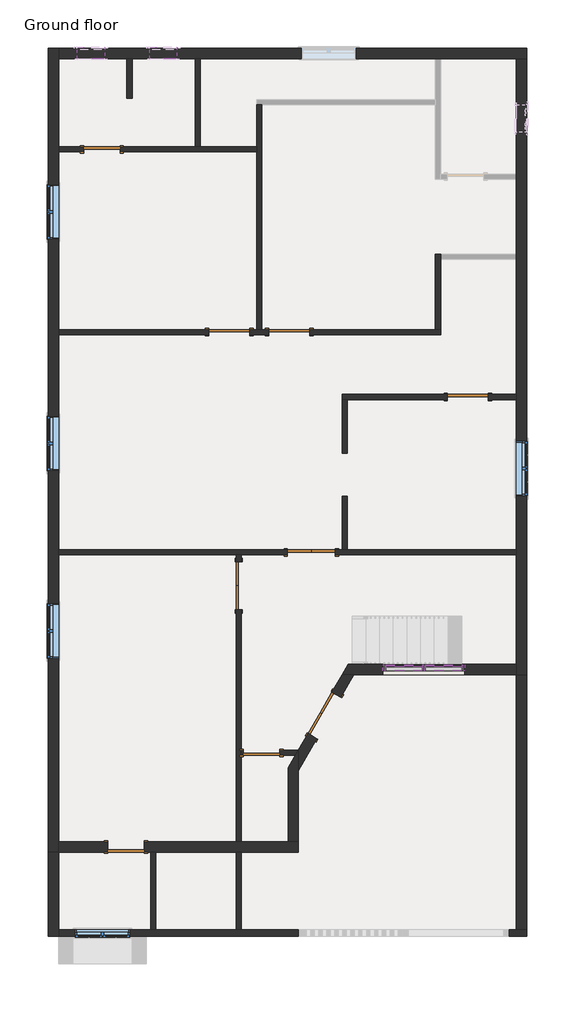
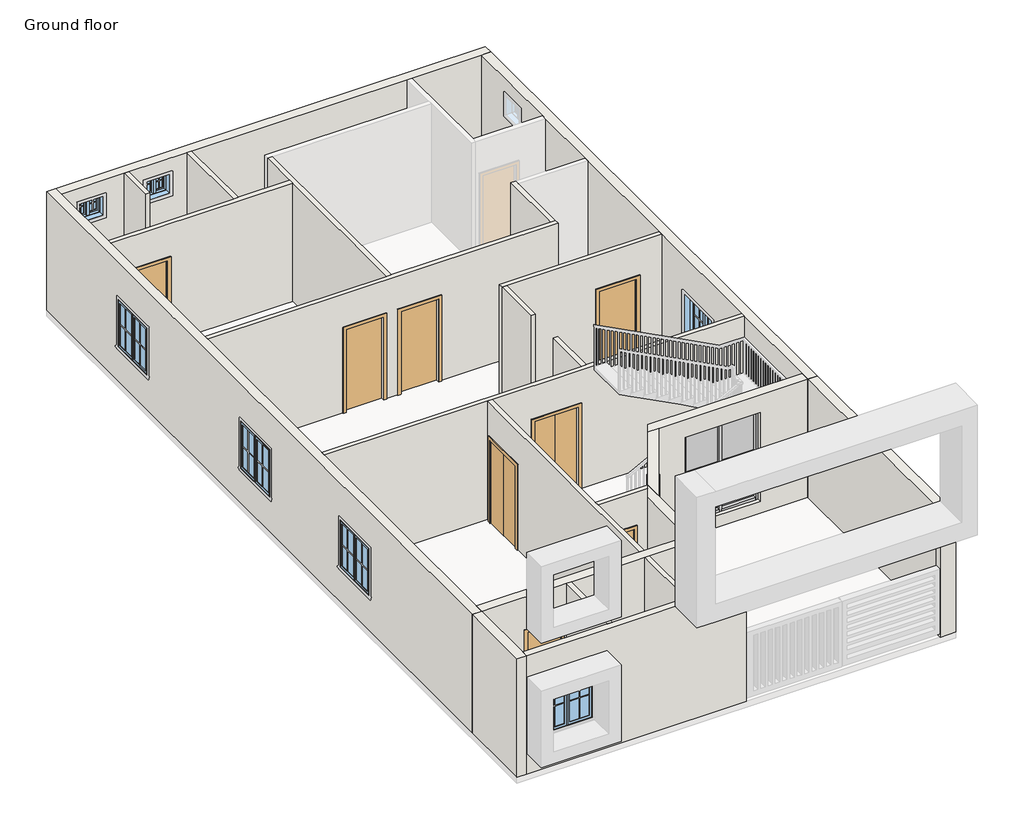
# One storey, part 1 of 3: 25 walls, 12 members, 9 doors, 7 windows, 4 plates.
"""IFC4 building model written with IfcOpenShell, lengths in millimetres."""

from ifc_helpers import new_model, si_unit, origin, origin_with_axes, place, context, project, spatial, polyline, outline, extrude, faceted_brep, transform, mapped, element, save
from components import door_d52489d9, door_d57fbbae, door_38851409, door_7b345704, single_flush_3_x7_e5f9f3c4, single_flush_3_x7_305aa2a5, member_c17f1be2, member_ad567e07, member_2b49869a, member_a715cb85, member_75074519, member_c4de40ee, system_panel_glazed_f4fd55f0, system_panel_glazed_231200ce, window_79894727, window_casement_double_4_x4_af3140d2, window_casement_double_4_x4_191d0cfb

model = new_model("IFC4")

# Units and contexts
model_context = context("Model", 3, world=origin())
ifc_project = project(units=[si_unit("LENGTHUNIT", "METRE", prefix="MILLI")], contexts=[model_context])

# Site, building, storey
site = spatial("IfcSite", under=ifc_project)
building = spatial("IfcBuilding", under=site)
storey = spatial("IfcBuildingStorey", under=building, Name="Ground floor", Elevation=0.0)

# Doors
placement = place(None, origin())
door_shape = door_d52489d9(model_context)
element("IfcDoor", 1, ObjectType="Door-Double-Flush_Panel : 3'6\"X7'", at=placement, inside=storey, context=model_context, shape_type="MappedRepresentation", body=[
    mapped(door_shape, transform((388.5194418, -4721.06525, 0.0), x_axis=(0.5010362705417002, 0.8654262854811288, 0.0), y_axis=(-0.8654262854811288, 0.5010362705417002, 0.0), z_axis=(0.0, 0.0, 1.0))),
])
door_2_shape = door_d57fbbae(model_context)
element("IfcDoor", 2, ObjectType="Door-Double-Flush_Panel : 3'6\"X7'", at=placement, inside=storey, context=model_context, shape_type="MappedRepresentation", body=[
    mapped(door_2_shape, transform((96.8585096, -1088.0023906, 0.0), x_axis=(1.0, 0.0, 0.0), y_axis=(0.0, 1.0, 0.0), z_axis=(0.0, 0.0, 1.0))),
])
element("IfcDoor", 3, ObjectType="Door-Double-Flush_Panel : 3'6\"X7'", at=placement, inside=storey, context=model_context, shape_type="MappedRepresentation", body=[
    mapped(door_2_shape, transform((-1522.3914904, -1830.9523906, 0.0), x_axis=(0.0, 1.0, 0.0), y_axis=(-1.0, 0.0, 0.0), z_axis=(0.0, 0.0, 1.0))),
])
door_3_shape = door_38851409(model_context)
element("IfcDoor", 4, ObjectType="Single-Flush : 2'8\"X7'", at=placement, inside=storey, context=model_context, shape_type="MappedRepresentation", body=[
    mapped(door_3_shape, transform((-1014.3914904, -5558.4023906, 0.0), x_axis=(1.0, 0.0, 0.0), y_axis=(0.0, 1.0, 0.0), z_axis=(0.0, 0.0, 1.0))),
])
element("IfcDoor", 5, ObjectType="Single-Flush : 2'8\"X7'", at=placement, inside=storey, context=model_context, shape_type="MappedRepresentation", body=[
    mapped(door_3_shape, transform((-4576.7414904, 7903.5976094, 0.0), x_axis=(-1.0, 0.0, 0.0), y_axis=(0.0, -1.0, 0.0), z_axis=(0.0, 0.0, 1.0))),
])
door_4_shape = door_7b345704(model_context)
element("IfcDoor", 6, ObjectType="Single-Flush : 2'8\"X7'", at=placement, inside=storey, context=model_context, shape_type="MappedRepresentation", body=[
    mapped(door_4_shape, transform((-4036.9914904, -7660.2523906, 0.0), x_axis=(1.0, 0.0, 0.0), y_axis=(0.0, 1.0, 0.0), z_axis=(0.0, 0.0, 1.0))),
])
single_flush_3_x7_shape = single_flush_3_x7_e5f9f3c4(model_context)
element("IfcDoor", 7, ObjectType="Single-Flush : 3'X7'", at=placement, inside=storey, context=model_context, shape_type="MappedRepresentation", body=[
    mapped(single_flush_3_x7_shape, transform((-1731.9414904, 3826.8976094, 0.0), x_axis=(1.0, 0.0, 0.0), y_axis=(0.0, 1.0, 0.0), z_axis=(0.0, 0.0, 1.0))),
])
single_flush_3_x7_2_shape = single_flush_3_x7_305aa2a5(model_context)
element("IfcDoor", 8, ObjectType="Single-Flush : 3'X7'", at=placement, inside=storey, context=model_context, shape_type="MappedRepresentation", body=[
    mapped(single_flush_3_x7_2_shape, transform((-398.4414904, 3826.8976094, 0.0), x_axis=(-1.0, 0.0, 0.0), y_axis=(0.0, -1.0, 0.0), z_axis=(0.0, 0.0, 1.0))),
])
element("IfcDoor", 9, ObjectType="Single-Flush : 3'X7'", at=placement, inside=storey, context=model_context, shape_type="MappedRepresentation", body=[
    mapped(single_flush_3_x7_2_shape, transform((3589.3585096, 2379.0976094, 0.0), x_axis=(-1.0, 0.0, 0.0), y_axis=(0.0, -1.0, 0.0), z_axis=(0.0, 0.0, 1.0))),
])

# Members
member_shape = member_c17f1be2(model_context)
element("IfcMember", 10, ObjectType="Rectangular Mullion : 2.5\" x 5\" rectangular", at=placement, inside=storey, context=model_context, shape_type="MappedRepresentation", body=[
    mapped(member_shape, transform((3456.0085096, -3659.7523906, 2590.8), x_axis=(0.0, 0.0, 1.0), y_axis=(0.0, -1.0, 0.0), z_axis=(1.0, 0.0, 0.0))),
])
element("IfcMember", 11, ObjectType="Rectangular Mullion : 2.5\" x 5\" rectangular", at=placement, inside=storey, context=model_context, shape_type="MappedRepresentation", body=[
    mapped(member_shape, transform((2573.3585096, -3659.7523906, 2590.8), x_axis=(0.0, 0.0, 1.0), y_axis=(0.0, -1.0, 0.0), z_axis=(1.0, 0.0, 0.0))),
])
element("IfcMember", 12, ObjectType="Rectangular Mullion : 2.5\" x 5\" rectangular", at=placement, inside=storey, context=model_context, shape_type="MappedRepresentation", body=[
    mapped(member_shape, transform((1754.2085096, -3659.7523906, 304.8), x_axis=(0.0, 0.0, -1.0), y_axis=(0.0, -1.0, 0.0), z_axis=(-1.0, 0.0, 0.0))),
])
element("IfcMember", 13, ObjectType="Rectangular Mullion : 2.5\" x 5\" rectangular", at=placement, inside=storey, context=model_context, shape_type="MappedRepresentation", body=[
    mapped(member_shape, transform((2636.8585096, -3659.7523906, 304.8), x_axis=(0.0, 0.0, -1.0), y_axis=(0.0, -1.0, 0.0), z_axis=(-1.0, 0.0, 0.0))),
])
member_2_shape = member_ad567e07(model_context)
element("IfcMember", 14, ObjectType="Rectangular Mullion : 2.5\" x 5\" rectangular", at=placement, inside=storey, context=model_context, shape_type="MappedRepresentation", body=[
    mapped(member_2_shape, transform((2573.3585096, -3659.7523906, 1524.0), x_axis=(0.0, 0.0, 1.0), y_axis=(0.0, -1.0, 0.0), z_axis=(1.0, 0.0, 0.0))),
])
element("IfcMember", 15, ObjectType="Rectangular Mullion : 2.5\" x 5\" rectangular", at=placement, inside=storey, context=model_context, shape_type="MappedRepresentation", body=[
    mapped(member_2_shape, transform((3456.0085096, -3659.7523906, 1524.0), x_axis=(0.0, 0.0, 1.0), y_axis=(0.0, -1.0, 0.0), z_axis=(1.0, 0.0, 0.0))),
])
member_3_shape = member_2b49869a(model_context)
element("IfcMember", 16, ObjectType="Rectangular Mullion : 2.5\" x 5\" rectangular", at=placement, inside=storey, context=model_context, shape_type="MappedRepresentation", body=[
    mapped(member_3_shape, transform((2605.1085096, -3659.7523906, 304.8), x_axis=(1.0, 0.0, 0.0), y_axis=(0.0, -1.0, 0.0), z_axis=(0.0, 0.0, -1.0))),
])
member_4_shape = member_a715cb85(model_context)
element("IfcMember", 17, ObjectType="Rectangular Mullion : 2.5\" x 5\" rectangular", at=placement, inside=storey, context=model_context, shape_type="MappedRepresentation", body=[
    mapped(member_4_shape, transform((2605.1085096, -3659.7523906, 1524.0), x_axis=(1.0, 0.0, 0.0), y_axis=(0.0, -1.0, 0.0), z_axis=(0.0, 0.0, -1.0))),
])
member_5_shape = member_75074519(model_context)
element("IfcMember", 18, ObjectType="Rectangular Mullion : 2.5\" x 5\" rectangular", at=placement, inside=storey, context=model_context, shape_type="MappedRepresentation", body=[
    mapped(member_5_shape, transform((3519.5085096, -3659.7523906, 304.8), x_axis=(1.0, 0.0, 0.0), y_axis=(0.0, -1.0, 0.0), z_axis=(0.0, 0.0, -1.0))),
])
member_6_shape = member_c4de40ee(model_context)
element("IfcMember", 19, ObjectType="Rectangular Mullion : 2.5\" x 5\" rectangular", at=placement, inside=storey, context=model_context, shape_type="MappedRepresentation", body=[
    mapped(member_6_shape, transform((1690.7085096, -3659.7523906, 2590.8), x_axis=(-1.0, 0.0, 0.0), y_axis=(0.0, -1.0, 0.0), z_axis=(0.0, 0.0, 1.0))),
])
element("IfcMember", 20, ObjectType="Rectangular Mullion : 2.5\" x 5\" rectangular", at=placement, inside=storey, context=model_context, shape_type="MappedRepresentation", body=[
    mapped(member_6_shape, transform((3519.5085096, -3659.7523906, 1524.0), x_axis=(1.0, 0.0, 0.0), y_axis=(0.0, -1.0, 0.0), z_axis=(0.0, 0.0, -1.0))),
])
element("IfcMember", 21, ObjectType="Rectangular Mullion : 2.5\" x 5\" rectangular", at=placement, inside=storey, context=model_context, shape_type="MappedRepresentation", body=[
    mapped(member_5_shape, transform((1690.7085096, -3659.7523906, 1524.0), x_axis=(-1.0, 0.0, 0.0), y_axis=(0.0, -1.0, 0.0), z_axis=(0.0, 0.0, 1.0))),
])

# Plates
system_panel_glazed_shape = system_panel_glazed_f4fd55f0(model_context)
element("IfcPlate", 22, ObjectType="System Panel : Glazed", at=placement, inside=storey, context=model_context, shape_type="MappedRepresentation", body=[
    mapped(system_panel_glazed_shape, transform((2163.7835096, -3659.7523906, 1555.75), x_axis=(1.0, 0.0, 0.0), y_axis=(0.0, 1.0, 0.0), z_axis=(0.0, 0.0, 1.0))),
])
element("IfcPlate", 23, ObjectType="System Panel : Glazed", at=placement, inside=storey, context=model_context, shape_type="MappedRepresentation", body=[
    mapped(system_panel_glazed_shape, transform((3046.4335096, -3659.7523906, 1555.75), x_axis=(1.0, 0.0, 0.0), y_axis=(0.0, 1.0, 0.0), z_axis=(0.0, 0.0, 1.0))),
])
system_panel_glazed_2_shape = system_panel_glazed_231200ce(model_context)
element("IfcPlate", 24, ObjectType="System Panel : Glazed", at=placement, inside=storey, context=model_context, shape_type="MappedRepresentation", body=[
    mapped(system_panel_glazed_2_shape, transform((2163.7835096, -3659.7523906, 368.3), x_axis=(1.0, 0.0, 0.0), y_axis=(0.0, 1.0, 0.0), z_axis=(0.0, 0.0, 1.0))),
])
element("IfcPlate", 25, ObjectType="System Panel : Glazed", at=placement, inside=storey, context=model_context, shape_type="MappedRepresentation", body=[
    mapped(system_panel_glazed_2_shape, transform((3046.4335096, -3659.7523906, 368.3), x_axis=(1.0, 0.0, 0.0), y_axis=(0.0, 1.0, 0.0), z_axis=(0.0, 0.0, 1.0))),
])

# Walls
element("IfcWall", 26, ObjectType="4.5\"", at=placement, inside=storey, context=model_context, shape_type="Brep", body=[
    faceted_brep([(-5543.5289904, 7846.4476094, 0.0), (-4983.1414904, 7846.4476094, 0.0), (-4983.1414904, 7846.4476094, 2133.6), (-4170.3414904, 7846.4476094, 2133.6), (-4170.3414904, 7846.4476094, 0.0), (-1122.3414904, 7846.4476094, 0.0), (-1122.3414904, 7846.4476094, 3048.0), (-5543.5289904, 7846.4476094, 3048.0), (-4983.1414904, 7960.7476094, 2133.6), (-4983.1414904, 7960.7476094, 0.0), (-5543.5289904, 7960.7476094, 0.0), (-5543.5289904, 7960.7476094, 3048.0), (-2493.9414904, 7960.7476094, 3048.0), (-2379.6414904, 7960.7476094, 3048.0), (-1122.3414904, 7960.7476094, 3048.0), (-1122.3414904, 7960.7476094, 0.0), (-2379.6414904, 7960.7476094, 0.0), (-2493.9414904, 7960.7476094, 0.0), (-4170.3414904, 7960.7476094, 0.0), (-4170.3414904, 7960.7476094, 2133.6)], [[[0, 1, 2, 3, 4, 5, 6, 7]], [[8, 9, 10, 11, 12, 13, 14, 15, 16, 17, 18, 19]], [[10, 9, 1, 0]], [[18, 17, 16, 15, 5, 4]], [[7, 6, 14, 13, 12, 11]], [[0, 7, 11, 10]], [[6, 5, 15, 14]], [[2, 1, 9, 8]], [[3, 2, 8, 19]], [[4, 3, 19, 18]]]),
])
element("IfcWall", 27, ObjectType="4.5\"", at=placement, inside=storey, context=model_context, shape_type="SweptSolid", body=[
    extrude(outline(polyline([(-2493.9414904, 7960.7476094), (-2493.9414904, 9929.2476094), (-2379.6414904, 9929.2476094), (-2379.6414904, 7960.7476094), (-2493.9414904, 7960.7476094)])), origin_with_axes(), (0.0, 0.0, 1.0), 3048.0),
])
element("IfcWall", 28, ObjectType="4.5\"", at=placement, inside=storey, context=model_context, shape_type="SweptSolid", body=[
    extrude(outline(polyline([(-4017.9414904, 9045.2567445), (-4017.9414904, 9929.2476094), (-3903.6414904, 9929.2476094), (-3903.6414904, 9045.2567445), (-4017.9414904, 9045.2567445)])), origin_with_axes(), (0.0, 0.0, 1.0), 3048.0),
])
element("IfcWall", 29, ObjectType="4.5\"", at=placement, inside=storey, context=model_context, shape_type="Brep", body=[
    faceted_brep([(-1274.7414904, 3769.7476094, 0.0), (-855.6414904, 3769.7476094, 0.0), (-855.6414904, 3769.7476094, 2133.6), (58.7585096, 3769.7476094, 2133.6), (58.7585096, 3769.7476094, 0.0), (2979.7585096, 3769.7476094, 0.0), (2979.7585096, 3769.7476094, 3048.0), (-5543.5289904, 3769.7476094, 3048.0), (-5543.5289904, 3769.7476094, 0.0), (-2189.1414904, 3769.7476094, 0.0), (-2189.1414904, 3769.7476094, 2133.6), (-1274.7414904, 3769.7476094, 2133.6), (-855.6414904, 3884.0476094, 2133.6), (-855.6414904, 3884.0476094, 0.0), (-1008.0414904, 3884.0476094, 0.0), (-1122.3414904, 3884.0476094, 0.0), (-1274.7414904, 3884.0476094, 0.0), (-1274.7414904, 3884.0476094, 2133.6), (-2189.1414904, 3884.0476094, 2133.6), (-2189.1414904, 3884.0476094, 0.0), (-5543.5289904, 3884.0476094, 0.0), (-5543.5289904, 3884.0476094, 3048.0), (-1122.3414904, 3884.0476094, 3048.0), (-1008.0414904, 3884.0476094, 3048.0), (2865.4585096, 3884.0476094, 3048.0), (2979.7585096, 3884.0476094, 3048.0), (2979.7585096, 3884.0476094, 0.0), (2865.4585096, 3884.0476094, 0.0), (58.7585096, 3884.0476094, 0.0), (58.7585096, 3884.0476094, 2133.6)], [[[0, 1, 2, 3, 4, 5, 6, 7, 8, 9, 10, 11]], [[12, 13, 14, 15, 16, 17, 18, 19, 20, 21, 22, 23, 24, 25, 26, 27, 28, 29]], [[9, 8, 20, 19]], [[28, 27, 26, 5, 4]], [[16, 15, 14, 13, 1, 0]], [[7, 6, 25, 24, 23, 22, 21]], [[8, 7, 21, 20]], [[6, 5, 26, 25]], [[17, 16, 0, 11]], [[18, 17, 11, 10]], [[19, 18, 10, 9]], [[2, 1, 13, 12]], [[3, 2, 12, 29]], [[4, 3, 29, 28]]]),
])
element("IfcWall", 30, ObjectType="4.5\"", at=placement, inside=storey, context=model_context, shape_type="Brep", body=[
    faceted_brep([(2979.7585096, 3884.0476094, 0.0), (2979.7585096, 5446.1476094, 0.0), (2979.7585096, 5560.4476094, 0.0), (2979.7585096, 5560.4476094, 3048.0), (2979.7585096, 5446.1476094, 3048.0), (2979.7585096, 3884.0476094, 3048.0), (2865.4585096, 3884.0476094, 0.0), (2865.4585096, 3884.0476094, 3048.0), (2865.4585096, 5560.4476094, 3048.0), (2865.4585096, 5560.4476094, 0.0)], [[[0, 1, 2, 3, 4, 5]], [[6, 7, 8, 9]], [[2, 1, 0, 6, 9]], [[5, 4, 3, 8, 7]], [[0, 5, 7, 6]], [[3, 2, 9, 8]]]),
])
element("IfcWall", 31, ObjectType="4.5\"", at=placement, inside=storey, context=model_context, shape_type="Brep", body=[
    faceted_brep([(3132.1585096, 2436.2476094, 2133.6), (3132.1585096, 2436.2476094, 0.0), (782.6585096, 2436.2476094, 0.0), (782.6585096, 2436.2476094, 3048.0), (4668.8585096, 2436.2476094, 3048.0), (4668.8585096, 2436.2476094, 0.0), (4046.5585096, 2436.2476094, 0.0), (4046.5585096, 2436.2476094, 2133.6), (782.6585096, 2321.9476094, 0.0), (896.9585096, 2321.9476094, 0.0), (3132.1585096, 2321.9476094, 0.0), (3132.1585096, 2321.9476094, 2133.6), (4046.5585096, 2321.9476094, 2133.6), (4046.5585096, 2321.9476094, 0.0), (4668.8585096, 2321.9476094, 0.0), (4668.8585096, 2321.9476094, 3048.0), (896.9585096, 2321.9476094, 3048.0), (782.6585096, 2321.9476094, 3048.0)], [[[0, 1, 2, 3, 4, 5, 6, 7]], [[8, 9, 10, 11, 12, 13, 14, 15, 16, 17]], [[6, 5, 14, 13]], [[2, 1, 10, 9, 8]], [[4, 3, 17, 16, 15]], [[5, 4, 15, 14]], [[3, 2, 8, 17]], [[11, 10, 1, 0]], [[12, 11, 0, 7]], [[13, 12, 7, 6]]]),
])
element("IfcWall", 32, ObjectType="4.5\"", at=placement, inside=storey, context=model_context, shape_type="SweptSolid", body=[
    extrude(outline(polyline([(782.6585096, 1121.7976094), (782.6585096, 2321.9476094), (896.9585096, 2321.9476094), (896.9585096, 1121.7976094), (782.6585096, 1121.7976094)])), origin_with_axes(), (0.0, 0.0, 1.0), 3048.0),
])
element("IfcWall", 33, ObjectType="4.5\"", at=placement, inside=storey, context=model_context, shape_type="Brep", body=[
    faceted_brep([(4668.8585096, -1145.1523906, 3048.0), (-1465.2414904, -1145.1523906, 3048.0), (-1579.5414904, -1145.1523906, 3048.0), (-5543.5289904, -1145.1523906, 3048.0), (-5543.5289904, -1145.1523906, 0.0), (-1579.5414904, -1145.1523906, 0.0), (-1465.2414904, -1145.1523906, 0.0), (-436.5414904, -1145.1523906, 0.0), (-436.5414904, -1145.1523906, 2133.6), (630.2585096, -1145.1523906, 2133.6), (630.2585096, -1145.1523906, 0.0), (4668.8585096, -1145.1523906, 0.0), (-5543.5289904, -1030.8523906, 3048.0), (782.6585096, -1030.8523906, 3048.0), (896.9585096, -1030.8523906, 3048.0), (4668.8585096, -1030.8523906, 3048.0), (4668.8585096, -1030.8523906, 0.0), (896.9585096, -1030.8523906, 0.0), (782.6585096, -1030.8523906, 0.0), (630.2585096, -1030.8523906, 0.0), (630.2585096, -1030.8523906, 2133.6), (-436.5414904, -1030.8523906, 2133.6), (-436.5414904, -1030.8523906, 0.0), (-5543.5289904, -1030.8523906, 0.0)], [[[0, 1, 2, 3, 4, 5, 6, 7, 8, 9, 10, 11]], [[12, 13, 14, 15, 16, 17, 18, 19, 20, 21, 22, 23]], [[4, 23, 22, 7, 6, 5]], [[16, 11, 10, 19, 18, 17]], [[3, 2, 1, 0, 15, 14, 13, 12]], [[4, 3, 12, 23]], [[0, 11, 16, 15]], [[9, 20, 19, 10]], [[20, 9, 8, 21]], [[21, 8, 7, 22]]]),
])
element("IfcWall", 34, ObjectType="4.5\"", at=placement, inside=storey, context=model_context, shape_type="Brep", body=[
    faceted_brep([(-1579.5414904, -7545.9523906, 3048.0), (-1579.5414904, -1145.1523906, 3048.0), (-1579.5414904, -1145.1523906, 0.0), (-1579.5414904, -1297.5523906, 0.0), (-1579.5414904, -1297.5523906, 2133.6), (-1579.5414904, -2364.3523906, 2133.6), (-1579.5414904, -2364.3523906, 0.0), (-1579.5414904, -7545.9523906, 0.0), (-1465.2414904, -1145.1523906, 3048.0), (-1465.2414904, -5501.2523906, 3048.0), (-1465.2414904, -5615.5523906, 3048.0), (-1465.2414904, -7545.9523906, 3048.0), (-1465.2414904, -7545.9523906, 0.0), (-1465.2414904, -5615.5523906, 0.0), (-1465.2414904, -5501.2523906, 0.0), (-1465.2414904, -2364.3523906, 0.0), (-1465.2414904, -2364.3523906, 2133.6), (-1465.2414904, -1297.5523906, 2133.6), (-1465.2414904, -1297.5523906, 0.0), (-1465.2414904, -1145.1523906, 0.0)], [[[0, 1, 2, 3, 4, 5, 6, 7]], [[8, 9, 10, 11, 12, 13, 14, 15, 16, 17, 18, 19]], [[2, 19, 18, 3]], [[12, 7, 6, 15, 14, 13]], [[1, 0, 11, 10, 9, 8]], [[0, 7, 12, 11]], [[2, 1, 8, 19]], [[17, 4, 3, 18]], [[4, 17, 16, 5]], [[5, 16, 15, 6]]]),
])
element("IfcWall", 35, ObjectType="4.5\"", at=placement, inside=storey, context=model_context, shape_type="Brep", body=[
    faceted_brep([(-607.9914904, -5615.5523906, 2133.6), (-607.9914904, -5615.5523906, 0.0), (-261.4151747, -5615.5523906, 0.0), (-261.4151747, -5615.5523906, 3048.0), (-1465.2414904, -5615.5523906, 3048.0), (-1465.2414904, -5615.5523906, 0.0), (-1420.7914904, -5615.5523906, 0.0), (-1420.7914904, -5615.5523906, 2133.6), (-195.2414904, -5501.2523906, 0.0), (-607.9914904, -5501.2523906, 0.0), (-607.9914904, -5501.2523906, 2133.6), (-1420.7914904, -5501.2523906, 2133.6), (-1420.7914904, -5501.2523906, 0.0), (-1465.2414904, -5501.2523906, 0.0), (-1465.2414904, -5501.2523906, 3048.0), (-195.2414904, -5501.2523906, 3048.0)], [[[0, 1, 2, 3, 4, 5, 6, 7]], [[8, 9, 10, 11, 12, 13, 14, 15]], [[6, 5, 13, 12]], [[2, 1, 9, 8]], [[4, 3, 15, 14]], [[3, 2, 8, 15]], [[5, 4, 14, 13]], [[10, 9, 1, 0]], [[11, 10, 0, 7]], [[12, 11, 7, 6]]]),
])
element("IfcWall", 36, ObjectType="4.5\"", at=placement, inside=storey, context=model_context, shape_type="Brep", body=[
    faceted_brep([(-1122.3414904, 8900.5476094, 0.0), (-1122.3414904, 7960.7476094, 0.0), (-1122.3414904, 7846.4476094, 0.0), (-1122.3414904, 3884.0476094, 0.0), (-1122.3414904, 3884.0476094, 3048.0), (-1122.3414904, 7846.4476094, 3048.0), (-1122.3414904, 7960.7476094, 3048.0), (-1122.3414904, 8900.5476094, 3048.0), (-1008.0414904, 8900.5476094, 0.0), (-1008.0414904, 8900.5476094, 3048.0), (-1008.0414904, 3884.0476094, 3048.0), (-1008.0414904, 3884.0476094, 0.0)], [[[0, 1, 2, 3, 4, 5, 6, 7]], [[8, 9, 10, 11]], [[3, 2, 1, 0, 8, 11]], [[7, 6, 5, 4, 10, 9]], [[0, 7, 9, 8]], [[4, 3, 11, 10]]]),
])
element("IfcWall", 37, ObjectType="4.5\"", at=placement, inside=storey, context=model_context, shape_type="SweptSolid", body=[
    extrude(outline(polyline([(-3484.5414904, -9501.7523906), (-3484.5414904, -7774.5523906), (-3370.2414904, -7774.5523906), (-3370.2414904, -9501.7523906), (-3484.5414904, -9501.7523906)])), origin_with_axes(), (0.0, 0.0, 1.0), 3048.0),
])
element("IfcWall", 38, ObjectType="4.5\"", at=placement, inside=storey, context=model_context, shape_type="SweptSolid", body=[
    extrude(outline(polyline([(-1579.5414904, -9501.7523906), (-1579.5414904, -7774.5523906), (-1465.2414904, -7774.5523906), (-1465.2414904, -9501.7523906), (-1579.5414904, -9501.7523906)])), origin_with_axes(), (0.0, 0.0, 1.0), 3048.0),
])
element("IfcWall", 39, ObjectType="4.5\"", at=placement, inside=storey, context=model_context, shape_type="SweptSolid", body=[
    extrude(outline(polyline([(782.6585096, -1030.8523906), (782.6585096, 169.2976094), (896.9585096, 169.2976094), (896.9585096, -1030.8523906), (782.6585096, -1030.8523906)])), origin_with_axes(), (0.0, 0.0, 1.0), 3048.0),
])
element("IfcWall", 40, ObjectType="6\"", at=placement, inside=storey, context=model_context, shape_type="Brep", body=[
    faceted_brep([(-5543.5289904, -9654.1523906, 0.0), (-195.2414904, -9654.1523906, 0.0), (-195.2414904, -9654.1523906, 3048.0), (-5543.5289904, -9654.1523906, 3048.0), (-5171.2602404, -9654.1523906, 2133.6), (-3952.0602404, -9654.1523906, 2133.6), (-3952.0602404, -9654.1523906, 914.4), (-5171.2602404, -9654.1523906, 914.4), (-5543.5289904, -9501.7523906, 0.0), (-5543.5289904, -9501.7523906, 3048.0), (-3484.5414904, -9501.7523906, 3048.0), (-3370.2414904, -9501.7523906, 3048.0), (-1579.5414904, -9501.7523906, 3048.0), (-1465.2414904, -9501.7523906, 3048.0), (-195.2414904, -9501.7523906, 3048.0), (-195.2414904, -9501.7523906, 0.0), (-1465.2414904, -9501.7523906, 0.0), (-1579.5414904, -9501.7523906, 0.0), (-3370.2414904, -9501.7523906, 0.0), (-3484.5414904, -9501.7523906, 0.0), (-5171.2602404, -9501.7523906, 2133.6), (-5171.2602404, -9501.7523906, 914.4), (-3952.0602404, -9501.7523906, 914.4), (-3952.0602404, -9501.7523906, 2133.6)], [[[0, 1, 2, 3], [4, 5, 6, 7]], [[8, 9, 10, 11, 12, 13, 14, 15, 16, 17, 18, 19], [20, 21, 22, 23]], [[1, 0, 8, 19, 18, 17, 16, 15]], [[2, 1, 15, 14]], [[3, 2, 14, 13, 12, 11, 10, 9]], [[0, 3, 9, 8]], [[21, 20, 4, 7]], [[22, 21, 7, 6]], [[23, 22, 6, 5]], [[20, 23, 5, 4]]]),
])
element("IfcWall", 41, ObjectType="6\"", at=placement, inside=storey, context=model_context, shape_type="Brep", body=[
    faceted_brep([(4897.4585096, -9501.7523906, 0.0), (4668.8585096, -9501.7523906, 0.0), (4516.4585096, -9501.7523906, 0.0), (4516.4585096, -9501.7523906, 3048.0), (4668.8585096, -9501.7523906, 3048.0), (4897.4585096, -9501.7523906, 3048.0), (4897.4585096, -9654.1523906, 0.0), (4897.4585096, -9654.1523906, 3048.0), (4516.4585096, -9654.1523906, 3048.0), (4516.4585096, -9654.1523906, 0.0)], [[[0, 1, 2, 3, 4, 5]], [[6, 7, 8, 9]], [[2, 1, 0, 6, 9]], [[3, 2, 9, 8]], [[5, 4, 3, 8, 7]], [[0, 5, 7, 6]]]),
])
element("IfcWall", 42, ObjectType="9\" 2", at=placement, inside=storey, context=model_context, shape_type="Brep", body=[
    faceted_brep([(-5772.1289904, 10157.8476094, 0.0), (-5772.1289904, -7774.5523906, 0.0), (-5772.1289904, -7774.5523906, 3048.0), (-5772.1289904, 10157.8476094, 3048.0), (-5772.1289904, 7117.9239079, 2133.6), (-5772.1289904, 5898.7239079, 2133.6), (-5772.1289904, 5898.7239079, 914.4), (-5772.1289904, 7117.9239079, 914.4), (-5772.1289904, 1953.7982391, 2133.6), (-5772.1289904, 734.5982391, 2133.6), (-5772.1289904, 734.5982391, 914.4), (-5772.1289904, 1953.7982391, 914.4), (-5772.1289904, -2229.9627914, 2133.6), (-5772.1289904, -3449.1627914, 2133.6), (-5772.1289904, -3449.1627914, 914.4), (-5772.1289904, -2229.9627914, 914.4), (-5543.5289904, 10157.8476094, 0.0), (-5543.5289904, 10157.8476094, 3048.0), (-5543.5289904, 9929.2476094, 3048.0), (-5543.5289904, 7960.7476094, 3048.0), (-5543.5289904, 7846.4476094, 3048.0), (-5543.5289904, 3884.0476094, 3048.0), (-5543.5289904, 3769.7476094, 3048.0), (-5543.5289904, -1030.8523906, 3048.0), (-5543.5289904, -1145.1523906, 3048.0), (-5543.5289904, -7545.9523906, 3048.0), (-5543.5289904, -7774.5523906, 3048.0), (-5543.5289904, -7774.5523906, 0.0), (-5543.5289904, -7545.9523906, 0.0), (-5543.5289904, -1145.1523906, 0.0), (-5543.5289904, -1030.8523906, 0.0), (-5543.5289904, 3769.7476094, 0.0), (-5543.5289904, 3884.0476094, 0.0), (-5543.5289904, 7846.4476094, 0.0), (-5543.5289904, 7960.7476094, 0.0), (-5543.5289904, 9929.2476094, 0.0), (-5543.5289904, 7117.9239079, 2133.6), (-5543.5289904, 7117.9239079, 914.4), (-5543.5289904, 5898.7239079, 914.4), (-5543.5289904, 5898.7239079, 2133.6), (-5543.5289904, 1953.7982391, 2133.6), (-5543.5289904, 1953.7982391, 914.4), (-5543.5289904, 734.5982391, 914.4), (-5543.5289904, 734.5982391, 2133.6), (-5543.5289904, -2229.9627914, 2133.6), (-5543.5289904, -2229.9627914, 914.4), (-5543.5289904, -3449.1627914, 914.4), (-5543.5289904, -3449.1627914, 2133.6)], [[[0, 1, 2, 3], [4, 5, 6, 7], [8, 9, 10, 11], [12, 13, 14, 15]], [[16, 17, 18, 19, 20, 21, 22, 23, 24, 25, 26, 27, 28, 29, 30, 31, 32, 33, 34, 35], [36, 37, 38, 39], [40, 41, 42, 43], [44, 45, 46, 47]], [[1, 0, 16, 35, 34, 33, 32, 31, 30, 29, 28, 27]], [[3, 2, 26, 25, 24, 23, 22, 21, 20, 19, 18, 17]], [[2, 1, 27, 26]], [[0, 3, 17, 16]], [[37, 36, 4, 7]], [[38, 37, 7, 6]], [[39, 38, 6, 5]], [[36, 39, 5, 4]], [[41, 40, 8, 11]], [[42, 41, 11, 10]], [[43, 42, 10, 9]], [[40, 43, 9, 8]], [[45, 44, 12, 15]], [[46, 45, 15, 14]], [[47, 46, 14, 13]], [[44, 47, 13, 12]]]),
])
element("IfcWall", 43, ObjectType="9\" 2", at=placement, inside=storey, context=model_context, shape_type="Brep", body=[
    faceted_brep([(-3630.5914904, -7774.5523906, 2133.6), (-3630.5914904, -7774.5523906, 0.0), (-3484.5414904, -7774.5523906, 0.0), (-3370.2414904, -7774.5523906, 0.0), (-1579.5414904, -7774.5523906, 0.0), (-1465.2414904, -7774.5523906, 0.0), (-195.2414904, -7774.5523906, 0.0), (-195.2414904, -7774.5523906, 3048.0), (-1465.2414904, -7774.5523906, 3048.0), (-1579.5414904, -7774.5523906, 3048.0), (-3370.2414904, -7774.5523906, 3048.0), (-3484.5414904, -7774.5523906, 3048.0), (-5543.5289904, -7774.5523906, 3048.0), (-5543.5289904, -7774.5523906, 0.0), (-4443.3914904, -7774.5523906, 0.0), (-4443.3914904, -7774.5523906, 2133.6), (-195.2414904, -7545.9523906, 0.0), (-423.8414904, -7545.9523906, 0.0), (-1465.2414904, -7545.9523906, 0.0), (-1579.5414904, -7545.9523906, 0.0), (-3630.5914904, -7545.9523906, 0.0), (-3630.5914904, -7545.9523906, 2133.6), (-4443.3914904, -7545.9523906, 2133.6), (-4443.3914904, -7545.9523906, 0.0), (-5543.5289904, -7545.9523906, 0.0), (-5543.5289904, -7545.9523906, 3048.0), (-1579.5414904, -7545.9523906, 3048.0), (-1465.2414904, -7545.9523906, 3048.0), (-423.8414904, -7545.9523906, 3048.0), (-195.2414904, -7545.9523906, 3048.0)], [[[0, 1, 2, 3, 4, 5, 6, 7, 8, 9, 10, 11, 12, 13, 14, 15]], [[16, 17, 18, 19, 20, 21, 22, 23, 24, 25, 26, 27, 28, 29]], [[14, 13, 24, 23]], [[6, 5, 4, 3, 2, 1, 20, 19, 18, 17, 16]], [[12, 11, 10, 9, 8, 7, 29, 28, 27, 26, 25]], [[13, 12, 25, 24]], [[7, 6, 16, 29]], [[21, 20, 1, 0]], [[22, 21, 0, 15]], [[23, 22, 15, 14]]]),
])
element("IfcWall", 44, ObjectType="9\" 2", at=placement, inside=storey, context=model_context, shape_type="Brep", body=[
    faceted_brep([(-195.2414904, -7545.9523906, 0.0), (-195.2414904, -5957.5067846, 0.0), (-195.2414904, -5501.2523906, 0.0), (-195.2414904, -5501.2523906, 3048.0), (-195.2414904, -5957.5067846, 3048.0), (-195.2414904, -7545.9523906, 3048.0), (-423.8414904, -7545.9523906, 0.0), (-423.8414904, -7545.9523906, 3048.0), (-423.8414904, -5896.106936, 3048.0), (-423.8414904, -5896.106936, 0.0), (-261.4151747, -5615.5523906, 0.0), (-261.4151747, -5615.5523906, 3048.0)], [[[0, 1, 2, 3, 4, 5]], [[6, 7, 8, 9]], [[2, 1, 0, 6, 9, 10]], [[5, 4, 3, 11, 8, 7]], [[0, 5, 7, 6]], [[3, 2, 10, 9, 8, 11]]]),
])
element("IfcWall", 45, ObjectType="9\" 2", at=placement, inside=storey, context=model_context, shape_type="Brep", body=[
    faceted_brep([(-5543.5289904, 9929.2476094, 0.0), (-4017.9414904, 9929.2476094, 0.0), (-3903.6414904, 9929.2476094, 0.0), (-2493.9414904, 9929.2476094, 0.0), (-2379.6414904, 9929.2476094, 0.0), (2865.4585096, 9929.2476094, 0.0), (2979.7585096, 9929.2476094, 0.0), (4668.8585096, 9929.2476094, 0.0), (4897.4585096, 9929.2476094, 0.0), (4897.4585096, 9929.2476094, 3048.0), (4668.8585096, 9929.2476094, 3048.0), (2979.7585096, 9929.2476094, 3048.0), (2865.4585096, 9929.2476094, 3048.0), (-2379.6414904, 9929.2476094, 3048.0), (-2493.9414904, 9929.2476094, 3048.0), (-3903.6414904, 9929.2476094, 3048.0), (-4017.9414904, 9929.2476094, 3048.0), (-5543.5289904, 9929.2476094, 3048.0), (-4512.8263632, 9929.2476094, 2667.0), (-4512.8263632, 9929.2476094, 2133.6), (-5122.4263632, 9929.2476094, 2133.6), (-5122.4263632, 9929.2476094, 2667.0), (-2900.8219932, 9929.2476094, 2667.0), (-2900.8219932, 9929.2476094, 2133.6), (-3510.4219932, 9929.2476094, 2133.6), (-3510.4219932, 9929.2476094, 2667.0), (1093.8085096, 9929.2476094, 2133.6), (1093.8085096, 9929.2476094, 914.4), (-125.3914904, 9929.2476094, 914.4), (-125.3914904, 9929.2476094, 2133.6), (-5543.5289904, 10157.8476094, 0.0), (-5543.5289904, 10157.8476094, 3048.0), (4897.4585096, 10157.8476094, 3048.0), (4897.4585096, 10157.8476094, 0.0), (-4512.8263632, 10157.8476094, 2667.0), (-5122.4263632, 10157.8476094, 2667.0), (-5122.4263632, 10157.8476094, 2133.6), (-4512.8263632, 10157.8476094, 2133.6), (-2900.8219932, 10157.8476094, 2667.0), (-3510.4219932, 10157.8476094, 2667.0), (-3510.4219932, 10157.8476094, 2133.6), (-2900.8219932, 10157.8476094, 2133.6), (1093.8085096, 10157.8476094, 2133.6), (-125.3914904, 10157.8476094, 2133.6), (-125.3914904, 10157.8476094, 914.4), (1093.8085096, 10157.8476094, 914.4)], [[[0, 1, 2, 3, 4, 5, 6, 7, 8, 9, 10, 11, 12, 13, 14, 15, 16, 17], [18, 19, 20, 21], [22, 23, 24, 25], [26, 27, 28, 29]], [[30, 31, 32, 33], [34, 35, 36, 37], [38, 39, 40, 41], [42, 43, 44, 45]], [[8, 7, 6, 5, 4, 3, 2, 1, 0, 30, 33]], [[17, 16, 15, 14, 13, 12, 11, 10, 9, 32, 31]], [[0, 17, 31, 30]], [[9, 8, 33, 32]], [[19, 18, 34, 37]], [[20, 19, 37, 36]], [[21, 20, 36, 35]], [[18, 21, 35, 34]], [[23, 22, 38, 41]], [[24, 23, 41, 40]], [[25, 24, 40, 39]], [[22, 25, 39, 38]], [[27, 26, 42, 45]], [[28, 27, 45, 44]], [[29, 28, 44, 43]], [[26, 29, 43, 42]]]),
])
element("IfcWall", 46, ObjectType="9\" 2", at=placement, inside=storey, context=model_context, shape_type="Brep", body=[
    faceted_brep([(4668.8585096, 9929.2476094, 0.0), (4668.8585096, 7351.1476094, 0.0), (4668.8585096, 7236.8476094, 0.0), (4668.8585096, 5560.4476094, 0.0), (4668.8585096, 5446.1476094, 0.0), (4668.8585096, 2436.2476094, 0.0), (4668.8585096, 2321.9476094, 0.0), (4668.8585096, -1030.8523906, 0.0), (4668.8585096, -1145.1523906, 0.0), (4668.8585096, -3583.5523906, 0.0), (4668.8585096, -3812.1523906, 0.0), (4668.8585096, -3824.8523906, 0.0), (4668.8585096, -3824.8523906, 3048.0), (4668.8585096, -3812.1523906, 3048.0), (4668.8585096, -3583.5523906, 3048.0), (4668.8585096, -1145.1523906, 3048.0), (4668.8585096, -1030.8523906, 3048.0), (4668.8585096, 2321.9476094, 3048.0), (4668.8585096, 2436.2476094, 3048.0), (4668.8585096, 5446.1476094, 3048.0), (4668.8585096, 5560.4476094, 3048.0), (4668.8585096, 7236.8476094, 3048.0), (4668.8585096, 7351.1476094, 3048.0), (4668.8585096, 9929.2476094, 3048.0), (4668.8585096, 172.8529692, 2133.6), (4668.8585096, 172.8529692, 914.4), (4668.8585096, 1392.0529692, 914.4), (4668.8585096, 1392.0529692, 2133.6), (4668.8585096, 8283.813041, 2667.0), (4668.8585096, 8283.813041, 2133.6), (4668.8585096, 8893.413041, 2133.6), (4668.8585096, 8893.413041, 2667.0), (4897.4585096, 9929.2476094, 0.0), (4897.4585096, 9929.2476094, 3048.0), (4897.4585096, -3824.8523906, 3048.0), (4897.4585096, -3824.8523906, 0.0), (4897.4585096, 172.8529692, 2133.6), (4897.4585096, 1392.0529692, 2133.6), (4897.4585096, 1392.0529692, 914.4), (4897.4585096, 172.8529692, 914.4), (4897.4585096, 8283.813041, 2667.0), (4897.4585096, 8893.413041, 2667.0), (4897.4585096, 8893.413041, 2133.6), (4897.4585096, 8283.813041, 2133.6)], [[[0, 1, 2, 3, 4, 5, 6, 7, 8, 9, 10, 11, 12, 13, 14, 15, 16, 17, 18, 19, 20, 21, 22, 23], [24, 25, 26, 27], [28, 29, 30, 31]], [[32, 33, 34, 35], [36, 37, 38, 39], [40, 41, 42, 43]], [[11, 10, 9, 8, 7, 6, 5, 4, 3, 2, 1, 0, 32, 35]], [[12, 11, 35, 34]], [[23, 22, 21, 20, 19, 18, 17, 16, 15, 14, 13, 12, 34, 33]], [[0, 23, 33, 32]], [[25, 24, 36, 39]], [[26, 25, 39, 38]], [[27, 26, 38, 37]], [[24, 27, 37, 36]], [[29, 28, 40, 43]], [[30, 29, 43, 42]], [[31, 30, 42, 41]], [[28, 31, 41, 40]]]),
])
element("IfcWall", 47, ObjectType="9\" 2", at=placement, inside=storey, context=model_context, shape_type="Brep", body=[
    faceted_brep([(4668.8585096, -3583.5523906, 0.0), (915.005878, -3583.5523906, 0.0), (915.005878, -3583.5523906, 3048.0), (4668.8585096, -3583.5523906, 3048.0), (1690.7085096, -3583.5523906, 2590.8), (1690.7085096, -3583.5523906, 304.8), (3519.5085096, -3583.5523906, 304.8), (3519.5085096, -3583.5523906, 2590.8), (782.6585096, -3812.1523906, 0.0), (1046.8057903, -3812.1523906, 0.0), (4668.8585096, -3812.1523906, 0.0), (4668.8585096, -3812.1523906, 3048.0), (1046.8057903, -3812.1523906, 3048.0), (782.6585096, -3812.1523906, 3048.0), (1690.7085096, -3812.1523906, 304.8), (1690.7085096, -3812.1523906, 2590.8), (3519.5085096, -3812.1523906, 2590.8), (3519.5085096, -3812.1523906, 304.8)], [[[0, 1, 2, 3], [4, 5, 6, 7]], [[8, 9, 10, 11, 12, 13], [14, 15, 16, 17]], [[1, 0, 10, 9, 8]], [[3, 2, 13, 12, 11]], [[0, 3, 11, 10]], [[2, 1, 8, 13]], [[14, 5, 4, 15]], [[15, 4, 7, 16]], [[16, 7, 6, 17]], [[5, 14, 17, 6]]]),
])
element("IfcWall", 48, ObjectType="9\" 2", at=placement, inside=storey, context=model_context, shape_type="Brep", body=[
    faceted_brep([(-195.2414904, -5501.2523906, 3048.0), (782.6585096, -3812.1523906, 3048.0), (782.6585096, -3812.1523906, 0.0), (556.8539641, -4202.1784236, 0.0), (556.8539641, -4202.1784236, 2133.6), (22.3484707, -5125.415185, 2133.6), (22.3484707, -5125.415185, 0.0), (-195.2414904, -5501.2523906, 0.0), (1046.8057903, -3812.1523906, 3048.0), (-195.2414904, -5957.5067846, 3048.0), (-195.2414904, -5957.5067846, 0.0), (220.1849195, -5239.9520764, 0.0), (220.1849195, -5239.9520764, 2133.6), (754.6904129, -4316.7153151, 2133.6), (754.6904129, -4316.7153151, 0.0), (1046.8057903, -3812.1523906, 0.0)], [[[0, 1, 2, 3, 4, 5, 6, 7]], [[8, 9, 10, 11, 12, 13, 14, 15]], [[2, 15, 14, 3]], [[10, 7, 6, 11]], [[1, 0, 9, 8]], [[2, 1, 8, 15]], [[0, 7, 10, 9]], [[13, 4, 3, 14]], [[4, 13, 12, 5]], [[5, 12, 11, 6]]]),
])
element("IfcWall", 49, ObjectType="9\" 2", at=placement, inside=storey, context=model_context, shape_type="Brep", body=[
    faceted_brep([(-5772.1289904, -7774.5523906, 0.0), (-5772.1289904, -9654.1523906, 0.0), (-5772.1289904, -9654.1523906, 3048.0), (-5772.1289904, -7774.5523906, 3048.0), (-5543.5289904, -7774.5523906, 0.0), (-5543.5289904, -7774.5523906, 3048.0), (-5543.5289904, -9501.7523906, 3048.0), (-5543.5289904, -9654.1523906, 3048.0), (-5543.5289904, -9654.1523906, 0.0), (-5543.5289904, -9501.7523906, 0.0)], [[[0, 1, 2, 3]], [[4, 5, 6, 7, 8, 9]], [[1, 0, 4, 9, 8]], [[3, 2, 7, 6, 5]], [[0, 3, 5, 4]], [[2, 1, 8, 7]]]),
])
element("IfcWall", 50, ObjectType="9\" 2", at=placement, inside=storey, context=model_context, shape_type="SweptSolid", body=[
    extrude(outline(polyline([(4668.8585096, -9501.7523906), (4668.8585096, -3824.8523906), (4897.4585096, -3824.8523906), (4897.4585096, -9501.7523906), (4668.8585096, -9501.7523906)])), origin_with_axes(), (0.0, 0.0, 1.0), 3048.0),
])

# Windows
window_shape = window_79894727(model_context)
element("IfcWindow", 51, ObjectType="Window-Casement-Double : 2'X1'9\"", at=placement, inside=storey, context=model_context, shape_type="MappedRepresentation", body=[
    mapped(window_shape, transform((-4817.6263632, 10043.5476094, 0.0), x_axis=(1.0, 0.0, 0.0), y_axis=(0.0, 1.0, 0.0), z_axis=(0.0, 0.0, 1.0))),
])
element("IfcWindow", 52, ObjectType="Window-Casement-Double : 2'X1'9\"", at=placement, inside=storey, context=model_context, shape_type="MappedRepresentation", body=[
    mapped(window_shape, transform((-3205.6219932, 10043.5476094, 0.0), x_axis=(1.0, 0.0, 0.0), y_axis=(0.0, 1.0, 0.0), z_axis=(0.0, 0.0, 1.0))),
])
window_casement_double_4_x4_shape = window_casement_double_4_x4_af3140d2(model_context)
element("IfcWindow", 53, ObjectType="Window-Casement-Double : 4'X4'", at=placement, inside=storey, context=model_context, shape_type="MappedRepresentation", body=[
    mapped(window_casement_double_4_x4_shape, transform((-5657.8289904, 6508.3239079, 0.0), x_axis=(0.0, 1.0, 0.0), y_axis=(-1.0, 0.0, 0.0), z_axis=(0.0, 0.0, 1.0))),
])
element("IfcWindow", 54, ObjectType="Window-Casement-Double : 4'X4'", at=placement, inside=storey, context=model_context, shape_type="MappedRepresentation", body=[
    mapped(window_casement_double_4_x4_shape, transform((-5657.8289904, 1344.1982391, 0.0), x_axis=(0.0, 1.0, 0.0), y_axis=(-1.0, 0.0, 0.0), z_axis=(0.0, 0.0, 1.0))),
])
element("IfcWindow", 55, ObjectType="Window-Casement-Double : 4'X4'", at=placement, inside=storey, context=model_context, shape_type="MappedRepresentation", body=[
    mapped(window_casement_double_4_x4_shape, transform((-5657.8289904, -2839.5627914, 0.0), x_axis=(0.0, 1.0, 0.0), y_axis=(-1.0, 0.0, 0.0), z_axis=(0.0, 0.0, 1.0))),
])
element("IfcWindow", 56, ObjectType="Window-Casement-Double : 4'X4'", at=placement, inside=storey, context=model_context, shape_type="MappedRepresentation", body=[
    mapped(window_casement_double_4_x4_shape, transform((4783.1585096, 782.4529692, 0.0), x_axis=(0.0, -1.0, 0.0), y_axis=(1.0, 0.0, 0.0), z_axis=(0.0, 0.0, 1.0))),
])
window_casement_double_4_x4_2_shape = window_casement_double_4_x4_191d0cfb(model_context)
element("IfcWindow", 57, ObjectType="Window-Casement-Double : 4'X4'", at=placement, inside=storey, context=model_context, shape_type="MappedRepresentation", body=[
    mapped(window_casement_double_4_x4_2_shape, transform((-4561.6602404, -9577.9523906, 0.0), x_axis=(-1.0, 0.0, 0.0), y_axis=(0.0, -1.0, 0.0), z_axis=(0.0, 0.0, 1.0))),
])

save(model, "model.ifc")

# Revit data of these elements
# Type "Door-Double-Flush_Panel : 3'6\"X7'"
#   Type Mark = "12"
#   Construction Type Id = "DOOR"
#   Assembly Code = "C1020"
#   Analytic Construction = "Wooden"
#   Thickness = 0' - 2"
#   Thermal Resistance (R) = 2.5876 (h·ft²·°F)/BTU
#   Swing Angle [instance default] = 90.00°
#   Panel Width = 1' - 9"
#   Heat Transfer Coefficient (U) = 0.3865 BTU/(h·ft²·°F)
#   Height = 7' - 0"
#   Trim Projection Ext = 0' - 1"
#   Trim Projection Int = 0' - 1"
#   Trim Width = 0' - 3"
#   Width = 3' - 6"
#   Define Thermal Properties by = 1
#   Panel Material = Wood - Birch - Solid Stained Light Low Gloss
#   Trim Material = Paint - Sienna
#   Visual Light Transmittance = 0
#   Solar Heat Gain Coefficient = 0
#   Function = (empty or 0)
#   Wall Closure = (empty or 0)
# Type "Single-Flush : 2'8\"X7'"
#   Type Mark = "9"
#   Construction Type Id = "MDOOR"
#   Assembly Code = "C1020"
#   Analytic Construction = "Metal"
#   Thickness = 0' - 2"
#   Heat Transfer Coefficient (U) = 0.651978 BTU/(h·ft²·°F)
#   Height = 7' - 0"
#   Trim Projection Ext = 0' - 1"
#   Trim Projection Int = 0' - 1"
#   Trim Width = 0' - 3"
#   Width = 2' - 8"
#   Define Thermal Properties by = 1
#   Door Material = Door - Panel
#   Frame Material = Door - Frame
#   Visual Light Transmittance = 0
#   Solar Heat Gain Coefficient = 0
#   Function = (empty or 0)
#   Wall Closure = (empty or 0)
# Type "Single-Flush : 3'X7'"
#   Type Mark = "8"
#   Construction Type Id = "MDOOR"
#   Assembly Code = "C1020"
#   Analytic Construction = "Metal"
#   Thickness = 0' - 2"
#   Heat Transfer Coefficient (U) = 0.651978 BTU/(h·ft²·°F)
#   Height = 7' - 0"
#   Trim Projection Ext = 0' - 1"
#   Trim Projection Int = 0' - 1"
#   Trim Width = 0' - 3"
#   Width = 3' - 0"
#   Define Thermal Properties by = 1
#   Door Material = Door - Panel
#   Frame Material = Door - Frame
#   Visual Light Transmittance = 0
#   Solar Heat Gain Coefficient = 0
#   Function = (empty or 0)
#   Wall Closure = (empty or 0)
# Type "Rectangular Mullion : 2.5\" x 5\" rectangular"
#   built-in parameter 1007304 = 0.416667 (stored number, unit not read)
#   built-in parameter 1007301 = 0.104167 (stored number, unit not read)
#   built-in parameter 1007300 = 0.104167 (stored number, unit not read)
# Type "System Panel : Glazed"
#   Construction Type Id = "GSP4R"
#   Analytic Construction = "1/8 in Pilkington single glazing"
#   Visual Light Transmittance = 0.9
#   Solar Heat Gain Coefficient = 0.86
#   Heat Transfer Coefficient (U) = 1.18115 BTU/(h·ft²·°F)
#   Define Thermal Properties by = 1
# Type "4.5\""
#   Assembly Code = "B2010"
#   Layers, outside or top first: 0' - 4 1/2" no material (function 1)
# Type "6\""
#   Assembly Code = "B2010"
#   Layers, outside or top first: 0' - 6" "wall 2" (function 1)
# Type "9\" 2"
#   Assembly Code = "B2010"
#   Layers, outside or top first: 0' - 9" "wall" (function 1)
# Type "Window-Casement-Double : 2'X1'9\""
#   Type Mark = "20"
#   Fire Rating = "0.5h"
#   Assembly Code = "B2020100"
#   Analytic Construction = "Double glazing - domestic"
#   Frame Extension [instance default] = 0' - 0 1/4"
#   Window Inset [instance default] = 0' - 0"
#   Wall Thickness [instance default] = 0' - 6"
#   Interior Wall Closure [instance default] = 0' - 2 1/4"
#   Half Width = 1' - 0"
#   Visual Light Transmittance = 0.81
#   Thermal Resistance (R) = 1.8146 (h·ft²·°F)/BTU
#   Solar Heat Gain Coefficient = 0.76
#   Rough Width = 2' - 0 1/2"
#   Rough Height = 1' - 9 1/2"
#   Height = 1' - 9"
#   Heat Transfer Coefficient (U) = 0.5511 BTU/(h·ft²·°F)
#   Exterior Wall Closure [instance default] = 0' - 1 1/4"
#   Extension Jamb [instance default] = 0' - 2 1/4"
#   Default Sill Height = 7' - 0"
#   Width = 2' - 0"
#   Muntin Visibility = yes
#   Interior Trim Visibility [instance default] = yes
#   Exterior Trim Visibility [instance default] = yes
#   Extension Jamb Visibility [instance default] = yes
#   Interior Trim Material = Wood - Stained
#   Muntin Pattern = Muntin Pattern_2x2 : Muntin Pattern_2x2
#   Interior Trim = Trim-Window-Interior-Flat : Picture Frame
#   Interior Frame Material = Wood - Stained
#   Glass Panel Material = Glass
#   Exterior Trim Material = Clad - White
#   Exterior Trim = Trim-Window-Exterior-Flat : with Sill
#   Exterior Frame Material = Clad - White
#   Wall Closure = (empty or 0)
# Type "Window-Casement-Double : 4'X4'"
#   Type Mark = "19"
#   Fire Rating = "0.5h"
#   Assembly Code = "B2020100"
#   Analytic Construction = "Double glazing - domestic"
#   Frame Extension [instance default] = 0' - 0 1/4"
#   Window Inset [instance default] = 0' - 0"
#   Wall Thickness [instance default] = 0' - 6"
#   Interior Wall Closure [instance default] = 0' - 2 1/4"
#   Half Width = 2' - 0"
#   Visual Light Transmittance = 0.81
#   Thermal Resistance (R) = 1.8146 (h·ft²·°F)/BTU
#   Solar Heat Gain Coefficient = 0.76
#   Rough Width = 4' - 0 1/2"
#   Rough Height = 4' - 0 1/2"
#   Height = 4' - 0"
#   Heat Transfer Coefficient (U) = 0.5511 BTU/(h·ft²·°F)
#   Exterior Wall Closure [instance default] = 0' - 1 1/4"
#   Extension Jamb [instance default] = 0' - 2 1/4"
#   Default Sill Height = 3' - 0"
#   Width = 4' - 0"
#   Muntin Visibility = yes
#   Interior Trim Visibility [instance default] = yes
#   Exterior Trim Visibility [instance default] = yes
#   Extension Jamb Visibility [instance default] = yes
#   Interior Trim Material = Wood - Stained
#   Muntin Pattern = Muntin Pattern_2x2 : Muntin Pattern_2x2
#   Interior Trim = Trim-Window-Interior-Flat : Picture Frame
#   Interior Frame Material = Wood - Stained
#   Glass Panel Material = Glass
#   Exterior Trim Material = Clad - White
#   Exterior Trim = Trim-Window-Exterior-Flat : with Sill
#   Exterior Frame Material = Clad - White
#   Wall Closure = (empty or 0)
# Elements 1, 2, 3 (IfcDoor, "Door-Double-Flush_Panel : 3'6\"X7'")
#   Swing Angle = 90.00°
#   Phase Created = New Construction
#   Materials on its faces: "Paint - Sienna", "Wood - Birch - Solid Stained Light Low Gloss"
# Elements 4, 5, 6 (IfcDoor, "Single-Flush : 2'8\"X7'")
#   Phase Created = New Construction
#   Materials on its faces: "Door - Frame", "Door - Panel"
# Elements 7, 8, 9 (IfcDoor, "Single-Flush : 3'X7'")
#   Phase Created = New Construction
#   Materials on its faces: "Door - Frame", "Door - Panel"
# Elements 10, 11, 12, 13, 14, 15, 16, 17, 18, 19, 20, 21 (IfcMember, "Rectangular Mullion : 2.5\" x 5\" rectangular")
#   Phase Created = New Construction
#   Materials on its faces: "Aluminum"
# Elements 22, 23, 24, 25 (IfcPlate, "System Panel : Glazed")
#   Phase Created = New Construction
#   Materials on its faces: "Glass"
# Elements 26, 27, 28, 29, 30, 31, 32, 33, 34, 35, 36, 37, 39 (IfcWall, "4.5\"")
#   Top Offset = -0' - 6"
#   Base Offset = 0' - 0"
#   wall height = 10' - 0"
#   Phase Created = New Construction
#   Base Constraint = Ground floor
#   Top Constraint = first floor
#   Materials on its faces: "Default Wall"
# Element 38 (IfcWall, "4.5\"")
#   Top Offset = -0' - 6"
#   Base Offset = 0' - 0"
#   wall height = 10' - 0"
#   Phase Created = New Construction
#   Base Constraint = Ground floor
#   Top Constraint = first floor
#   Materials on its faces: "Default Wall", "wall 1"
# Element 40 (IfcWall, "6\"")
#   Top Offset = -0' - 6"
#   Base Offset = 0' - 0"
#   wall height = 10' - 0"
#   Phase Created = New Construction
#   Base Constraint = Ground floor
#   Top Constraint = first floor
#   Materials on its faces: "wall 2", "wall 1"
# Element 41 (IfcWall, "6\"")
#   Top Offset = -0' - 6"
#   Base Offset = 0' - 0"
#   wall height = 10' - 0"
#   Phase Created = New Construction
#   Base Constraint = Ground floor
#   Top Constraint = first floor
#   Materials on its faces: "wall 2", "6\" wall"
# Elements 42, 45 (IfcWall, "9\" 2")
#   Top Offset = -0' - 6"
#   Base Offset = 0' - 0"
#   wall height = 10' - 0"
#   Phase Created = New Construction
#   Base Constraint = Ground floor
#   Top Constraint = first floor
#   Materials on its faces: "wall", "wall 1", "6\" wall"
# Elements 43, 44, 48 (IfcWall, "9\" 2")
#   Top Offset = -0' - 6"
#   Base Offset = 0' - 0"
#   wall height = 10' - 0"
#   Phase Created = New Construction
#   Base Constraint = Ground floor
#   Top Constraint = first floor
#   Materials on its faces: "wall", "wall 1"
# Elements 46, 47, 50 (IfcWall, "9\" 2")
#   Top Offset = -0' - 6"
#   Base Offset = 0' - 0"
#   wall height = 10' - 0"
#   Phase Created = New Construction
#   Base Constraint = Ground floor
#   Top Constraint = first floor
#   Materials on its faces: "wall", "6\" wall"
# Element 49 (IfcWall, "9\" 2")
#   Top Offset = -0' - 6"
#   Base Offset = 0' - 0"
#   wall height = 10' - 0"
#   Phase Created = New Construction
#   Base Constraint = Ground floor
#   Top Constraint = first floor
#   Materials on its faces: "wall", "6\" wall", "wall 1"
# Element 51 (IfcWindow, "Window-Casement-Double : 2'X1'9\"")
#   Mark = "5"
#   Window Inset = 0' - 0"
#   Interior Wall Closure = 0' - 2 1/4"
#   Frame Extension = 0' - 0 1/4"
#   Exterior Wall Closure = 0' - 1 1/4"
#   Interior Trim Visibility = yes
#   Exterior Trim Visibility = yes
#   Phase Created = New Construction
#   Materials on its faces: "Wood - Stained", "Glass", "Clad - White"
# Element 52 (IfcWindow, "Window-Casement-Double : 2'X1'9\"")
#   Mark = "6"
#   Window Inset = 0' - 0"
#   Interior Wall Closure = 0' - 2 1/4"
#   Frame Extension = 0' - 0 1/4"
#   Exterior Wall Closure = 0' - 1 1/4"
#   Interior Trim Visibility = yes
#   Exterior Trim Visibility = yes
#   Phase Created = New Construction
#   Materials on its faces: "Wood - Stained", "Glass", "Clad - White"
# Element 53 (IfcWindow, "Window-Casement-Double : 4'X4'")
#   Mark = "1"
#   Window Inset = 0' - 0"
#   Interior Wall Closure = 0' - 2 1/4"
#   Frame Extension = 0' - 0 1/4"
#   Exterior Wall Closure = 0' - 1 1/4"
#   Interior Trim Visibility = yes
#   Exterior Trim Visibility = yes
#   Phase Created = New Construction
#   Materials on its faces: "Wood - Stained", "Glass", "Clad - White"
# Element 54 (IfcWindow, "Window-Casement-Double : 4'X4'")
#   Mark = "2"
#   Window Inset = 0' - 0"
#   Interior Wall Closure = 0' - 2 1/4"
#   Frame Extension = 0' - 0 1/4"
#   Exterior Wall Closure = 0' - 1 1/4"
#   Interior Trim Visibility = yes
#   Exterior Trim Visibility = yes
#   Phase Created = New Construction
#   Materials on its faces: "Wood - Stained", "Glass", "Clad - White"
# Element 55 (IfcWindow, "Window-Casement-Double : 4'X4'")
#   Mark = "3"
#   Window Inset = 0' - 0"
#   Interior Wall Closure = 0' - 2 1/4"
#   Frame Extension = 0' - 0 1/4"
#   Exterior Wall Closure = 0' - 1 1/4"
#   Interior Trim Visibility = yes
#   Exterior Trim Visibility = yes
#   Phase Created = New Construction
#   Materials on its faces: "Wood - Stained", "Glass", "Clad - White"
# Element 56 (IfcWindow, "Window-Casement-Double : 4'X4'")
#   Mark = "4"
#   Window Inset = 0' - 0"
#   Interior Wall Closure = 0' - 2 1/4"
#   Frame Extension = 0' - 0 1/4"
#   Exterior Wall Closure = 0' - 1 1/4"
#   Interior Trim Visibility = yes
#   Exterior Trim Visibility = yes
#   Phase Created = New Construction
#   Materials on its faces: "Wood - Stained", "Glass", "Clad - White"
# Element 57 (IfcWindow, "Window-Casement-Double : 4'X4'")
#   Mark = "8"
#   Window Inset = 0' - 0"
#   Interior Wall Closure = 0' - 2 1/4"
#   Frame Extension = 0' - 0 1/4"
#   Exterior Wall Closure = 0' - 1 1/4"
#   Interior Trim Visibility = yes
#   Exterior Trim Visibility = yes
#   Phase Created = New Construction
#   Materials on its faces: "Wood - Stained", "Glass", "Clad - White"
# Materials
#   "Wood - Birch - Solid Stained Light Low Gloss": class "Wood", colour RGB 210 159 95, transparency 0, Cost = 0
#   "Paint - Sienna": colour RGB 118 70 51, transparency 0, Cost = 0
#   "Door - Panel": class "Wood", colour RGB 210 159 95, transparency 0, Cost = 0
#   "Door - Frame": colour RGB 118 70 51, transparency 0, Cost = 0
#   "wall 2": class "Generic", colour RGB 34 30 27, transparency 0, Cost = 0
#   "wall": class "Generic", colour RGB 93 108 103, transparency 0, Cost = 0
#   "Wood - Stained": class "Wood", colour RGB 224 178 126, transparency 0, Cost = 0
#   "Glass": class "Glass", colour RGB 0 128 192, transparency 0.75, Description = "Soda Lime Glass", Cost = 0
#   "Clad - White": class "Wood", colour RGB 242 242 238, transparency 0, Cost = 0
#   "Aluminum": class "Metal", colour RGB 247 247 247, transparency 0, Description = "Aluminum 6061", Cost = 0
#   "Default Wall": colour RGB 128 128 128, transparency 0, Cost = 0
#   "wall 1": class "Generic", colour RGB 133 142 137, transparency 0, Cost = 0
#   "6\" wall": class "Generic", colour RGB 136 79 68, transparency 0, Cost = 0
